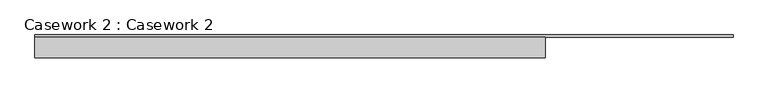
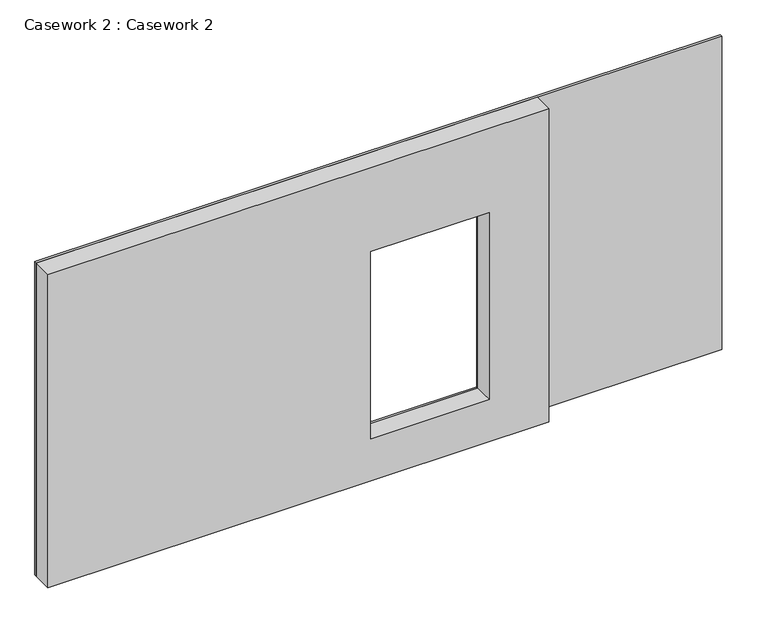
"""IFC4 building model written with IfcOpenShell, lengths in millimetres: furniture geometry, Casework 2 : Casework 2."""

from ifc_helpers import new_model, si_unit, frame, origin, place, context, project, spatial, polyline, outline, extrude, source, transform, mapped, element, save


def casework_2_casework_2_9c5fcee0(model_context):
    return source(origin(), model_context, "Body", "SweptSolid", [
        extrude(outline(polyline([(7600.0, -15625.2520625), (7600.0, -20687.7520625), (4250.0, -20687.7520625), (4250.0, -15625.2520625), (7600.0, -15625.2520625)]), holes=[polyline([(6700.0, -16225.2520625), (4700.0, -16225.2520625), (4700.0, -17425.2520625), (6700.0, -17425.2520625), (6700.0, -16225.2520625)])]), frame((0.0, -10451.0480844, 0.0), z_axis=(0.0, 1.0, 0.0), x_axis=(0.0, 0.0, 1.0)), (0.0, 0.0, 1.0), 200.0),
        extrude(outline(polyline([(7600.0, -13762.7520625), (7600.0, -20687.7520625), (4250.0, -20687.7520625), (4250.0, -13762.7520625), (7600.0, -13762.7520625)]), holes=[polyline([(6700.0, -16225.2520625), (4700.0, -16225.2520625), (4700.0, -17425.2520625), (6700.0, -17425.2520625), (6700.0, -16225.2520625)])]), frame((0.0, -10251.0480844, 0.0), z_axis=(0.0, 1.0, 0.0), x_axis=(0.0, 0.0, 1.0)), (0.0, 0.0, 1.0), 25.0),
    ])


if __name__ == "__main__":
    model = new_model("IFC4")
    model_context = context("Model", 3, world=origin())
    ifc_project = project(units=[si_unit("LENGTHUNIT", "METRE", prefix="MILLI")], contexts=[model_context])
    site = spatial("IfcSite", under=ifc_project)
    building = spatial("IfcBuilding", under=site)
    placement = place(None, origin())
    casework_2_casework_2_shape = casework_2_casework_2_9c5fcee0(model_context)
    element("IfcFurniture", 1, ObjectType="Casework 2 : Casework 2", at=placement, inside=building, context=model_context, shape_type="MappedRepresentation", body=[
        mapped(casework_2_casework_2_shape, transform((0.0, 0.0, 0.0), x_axis=(1.0, 0.0, 0.0), y_axis=(0.0, 1.0, 0.0), z_axis=(0.0, 0.0, 1.0))),
    ])
    save(model, "model.ifc")

# Revit data of these elements
# Element 1 (IfcFurniture, "Casework 2 : Casework 2")
#   Materials on its faces: "Wood Door Panel - Birch", "wood ext"
# Materials
#   "Wood Door Panel - Birch": class "Wood", colour RGB 166 116 52, transparency 0
#   "wood ext": class "Generic", colour RGB 91 21 0, transparency 0, Cost = 0
